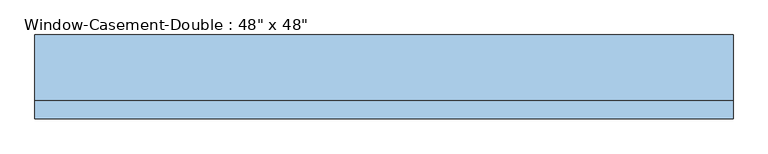
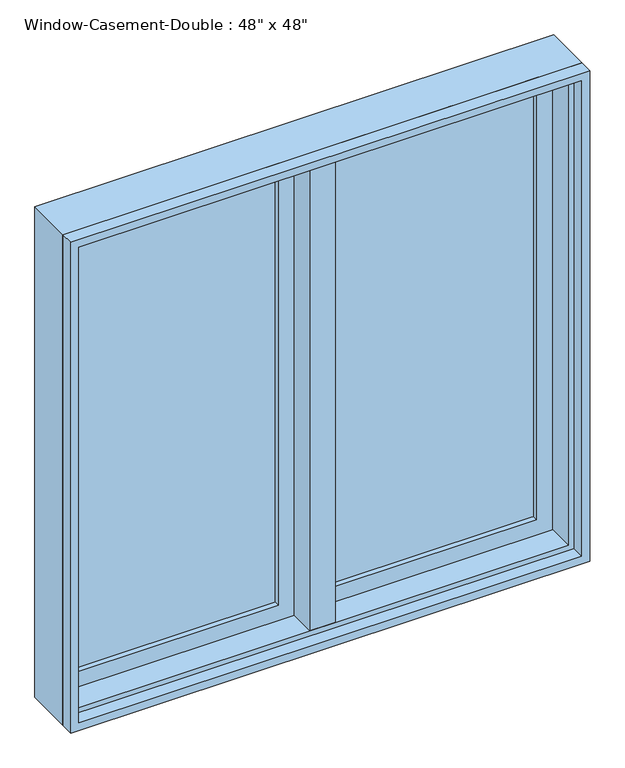
"""IFC4 building model written with IfcOpenShell, lengths in millimetres: window geometry."""

from ifc_helpers import new_model, si_unit, frame, origin, place, context, project, spatial, polyline, outline, extrude, faceted_brep, source, transform, mapped, element, save


def window_c2c97eee(model_context):
    return source(origin(), model_context, "Body", "SolidModel", [
        faceted_brep([(577.85, 31.75, 2101.85), (577.85, -31.75, 2101.85), (-577.85, -31.75, 2101.85), (-577.85, 31.75, 2101.85), (596.9, 82.55, 2120.9), (596.9, 31.75, 2120.9), (-596.9, 31.75, 2120.9), (-596.9, 82.55, 2120.9), (609.6, -31.75, 2133.6), (609.6, 82.55, 2133.6), (-609.6, 82.55, 2133.6), (-609.6, -31.75, 2133.6), (-577.85, -31.75, 946.15), (-577.85, 31.75, 946.15), (-596.9, 31.75, 927.1), (-596.9, 82.55, 927.1), (-609.6, 82.55, 914.4), (-609.6, -31.75, 914.4), (577.85, -31.75, 946.15), (577.85, 31.75, 946.15), (596.9, 31.75, 927.1), (596.9, 82.55, 927.1), (609.6, 82.55, 914.4), (609.6, -31.75, 914.4)], [[[0, 1, 2, 3]], [[4, 5, 6, 7]], [[8, 9, 10, 11]], [[3, 2, 12, 13]], [[7, 6, 14, 15]], [[11, 10, 16, 17]], [[13, 12, 18, 19]], [[15, 14, 20, 21]], [[17, 16, 22, 23]], [[11, 17, 23, 8], [1, 18, 12, 2]], [[19, 18, 1, 0]], [[5, 20, 14, 6], [3, 13, 19, 0]], [[21, 20, 5, 4]], [[23, 22, 9, 8]], [[9, 22, 16, 10], [7, 15, 21, 4]]]),
        extrude(outline(polyline([(2133.6, -609.6), (914.4, -609.6), (914.4, 609.6), (2133.6, 609.6), (2133.6, -609.6)]), holes=[polyline([(2114.55, 590.55), (933.45, 590.55), (933.45, -590.55), (2114.55, -590.55), (2114.55, 590.55)])]), frame((0.0, -63.5, 0.0), z_axis=(0.0, 1.0, 0.0), x_axis=(0.0, 0.0, 1.0)), (0.0, 0.0, 1.0), 31.75),
        extrude(outline(polyline([(927.1, 596.9), (2120.9, 596.9), (2120.9, 9.525), (927.1, 9.525), (927.1, 596.9)]), holes=[polyline([(984.25, 66.675), (2063.75, 66.675), (2063.75, 539.75), (984.25, 539.75), (984.25, 66.675)])]), frame((0.0, 31.75, 0.0), z_axis=(0.0, 1.0, 0.0), x_axis=(0.0, 0.0, 1.0)), (0.0, 0.0, 1.0), 44.45),
        extrude(outline(polyline([(2120.9, -596.9), (927.1, -596.9), (927.1, -9.525), (2120.9, -9.525), (2120.9, -596.9)]), holes=[polyline([(2063.75, -66.675), (984.25, -66.675), (984.25, -539.75), (2063.75, -539.75), (2063.75, -66.675)])]), frame((0.0, 31.75, 0.0), z_axis=(0.0, 1.0, 0.0), x_axis=(0.0, 0.0, 1.0)), (0.0, 0.0, 1.0), 44.45),
        extrude(outline(polyline([(539.75, 63.5), (539.75, 57.15), (66.675, 57.15), (66.675, 63.5), (539.75, 63.5)])), frame((0.0, 0.0, 984.25), z_axis=(0.0, 0.0, 1.0), x_axis=(1.0, 0.0, 0.0)), (0.0, 0.0, 1.0), 1079.5),
        extrude(outline(polyline([(66.675, 44.45), (66.675, 50.8), (539.75, 50.8), (539.75, 44.45), (66.675, 44.45)])), frame((0.0, 0.0, 984.25), z_axis=(0.0, 0.0, 1.0), x_axis=(1.0, 0.0, 0.0)), (0.0, 0.0, 1.0), 1079.5),
        extrude(outline(polyline([(-66.675, 63.5), (-66.675, 57.15), (-539.75, 57.15), (-539.75, 63.5), (-66.675, 63.5)])), frame((0.0, 0.0, 984.25), z_axis=(0.0, 0.0, 1.0), x_axis=(1.0, 0.0, 0.0)), (0.0, 0.0, 1.0), 1079.5),
        extrude(outline(polyline([(-539.75, 44.45), (-539.75, 50.8), (-66.675, 50.8), (-66.675, 44.45), (-539.75, 44.45)])), frame((0.0, 0.0, 984.25), z_axis=(0.0, 0.0, 1.0), x_axis=(1.0, 0.0, 0.0)), (0.0, 0.0, 1.0), 1079.5),
        faceted_brep([(9.525, 82.55, 2120.9), (-9.525, 82.55, 2120.9), (-9.525, 31.75, 2120.9), (9.525, 31.75, 2120.9), (9.525, 82.55, 927.1), (9.525, 31.75, 927.1), (-9.525, 31.75, 927.1), (-9.525, 82.55, 927.1), (-9.525, 31.75, 946.15), (-9.525, 31.75, 2101.85), (-30.1625, 31.75, 946.15), (-30.1625, 31.75, 2101.85), (-30.1625, -31.75, 946.15), (-30.1625, -31.75, 2101.85), (30.1625, -31.75, 946.15), (30.1625, -31.75, 2101.85), (30.1625, 31.75, 946.15), (30.1625, 31.75, 2101.85), (9.525, 31.75, 946.15), (9.525, 31.75, 2101.85)], [[[0, 1, 2, 3]], [[4, 5, 6, 7]], [[1, 0, 4, 7]], [[2, 1, 7, 6, 8, 9]], [[9, 8, 10, 11]], [[11, 10, 12, 13]], [[13, 12, 14, 15]], [[15, 14, 16, 17]], [[17, 16, 18, 19]], [[0, 3, 19, 18, 5, 4]], [[18, 8, 6, 5]], [[9, 19, 3, 2]], [[8, 18, 16, 14, 12, 10]], [[19, 9, 11, 13, 15, 17]]]),
    ])


if __name__ == "__main__":
    model = new_model("IFC4")
    model_context = context("Model", 3, world=origin())
    ifc_project = project(units=[si_unit("LENGTHUNIT", "METRE", prefix="MILLI")], contexts=[model_context])
    site = spatial("IfcSite", under=ifc_project)
    building = spatial("IfcBuilding", under=site)
    placement = place(None, origin())
    window_shape = window_c2c97eee(model_context)
    element("IfcWindow", 1, ObjectType="Window-Casement-Double : 48\" x 48\"", at=placement, inside=building, context=model_context, shape_type="MappedRepresentation", body=[
        mapped(window_shape, transform((0.0, 0.0, 0.0), x_axis=(1.0, 0.0, 0.0), y_axis=(0.0, 1.0, 0.0), z_axis=(0.0, 0.0, 1.0))),
    ])
    save(model, "model.ifc")

# Revit data of these elements
# Type "Window-Casement-Double : 48\" x 48\""
#   Type Mark = "18"
#   Fire Rating = "0.5h"
#   Assembly Code = "B2020100"
#   Analytic Construction = "Double glazing - domestic"
#   Frame Extension [instance default] = 0' - 0 1/4"
#   Window Inset [instance default] = 0' - 0"
#   Wall Thickness [instance default] = 0' - 6"
#   Interior Wall Closure [instance default] = 0' - 2 1/4"
#   Half Width = 2' - 0"
#   Visual Light Transmittance = 0.81
#   Thermal Resistance (R) = 1.8146 (h·ft²·°F)/BTU
#   Solar Heat Gain Coefficient = 0.76
#   Rough Width = 4' - 0 1/2"
#   Rough Height = 4' - 0 1/2"
#   Height = 4' - 0"
#   Heat Transfer Coefficient (U) = 0.5511 BTU/(h·ft²·°F)
#   Exterior Wall Closure [instance default] = 0' - 1 1/4"
#   Extension Jamb [instance default] = 0' - 2 1/4"
#   Default Sill Height = 3' - 0"
#   Width = 4' - 0"
#   Muntin Visibility = yes
#   Interior Trim Visibility [instance default] = yes
#   Exterior Trim Visibility [instance default] = yes
#   Extension Jamb Visibility [instance default] = yes
#   Interior Trim Material = Wood - Stained
#   Muntin Pattern = Muntin Pattern_2x2 : Muntin Pattern_2x2
#   Interior Trim = Trim-Window-Interior-Flat : Picture Frame
#   Interior Frame Material = Wood - Stained
#   Glass Panel Material = Glass
#   Exterior Trim Material = Clad - White
#   Exterior Trim = Trim-Window-Exterior-Flat : with Sill
#   Exterior Frame Material = Clad - White
#   Wall Closure = (empty or 0)
# Element 1 (IfcWindow, "Window-Casement-Double : 48\" x 48\"")
#   Wall Thickness = 0' - 5"
#   Extension Jamb = 0' - 1 1/4"
#   Materials on its faces: "Wood - Stained", "Glass", "Clad - White"
# Materials
#   "Wood - Stained": class "Wood", colour RGB 224 178 126, transparency 0, Cost = 0
#   "Glass": class "Glass", colour RGB 0 128 192, transparency 0.75, Description = "Soda Lime Glass", Cost = 0
#   "Clad - White": class "Wood", colour RGB 242 242 238, transparency 0, Cost = 0
